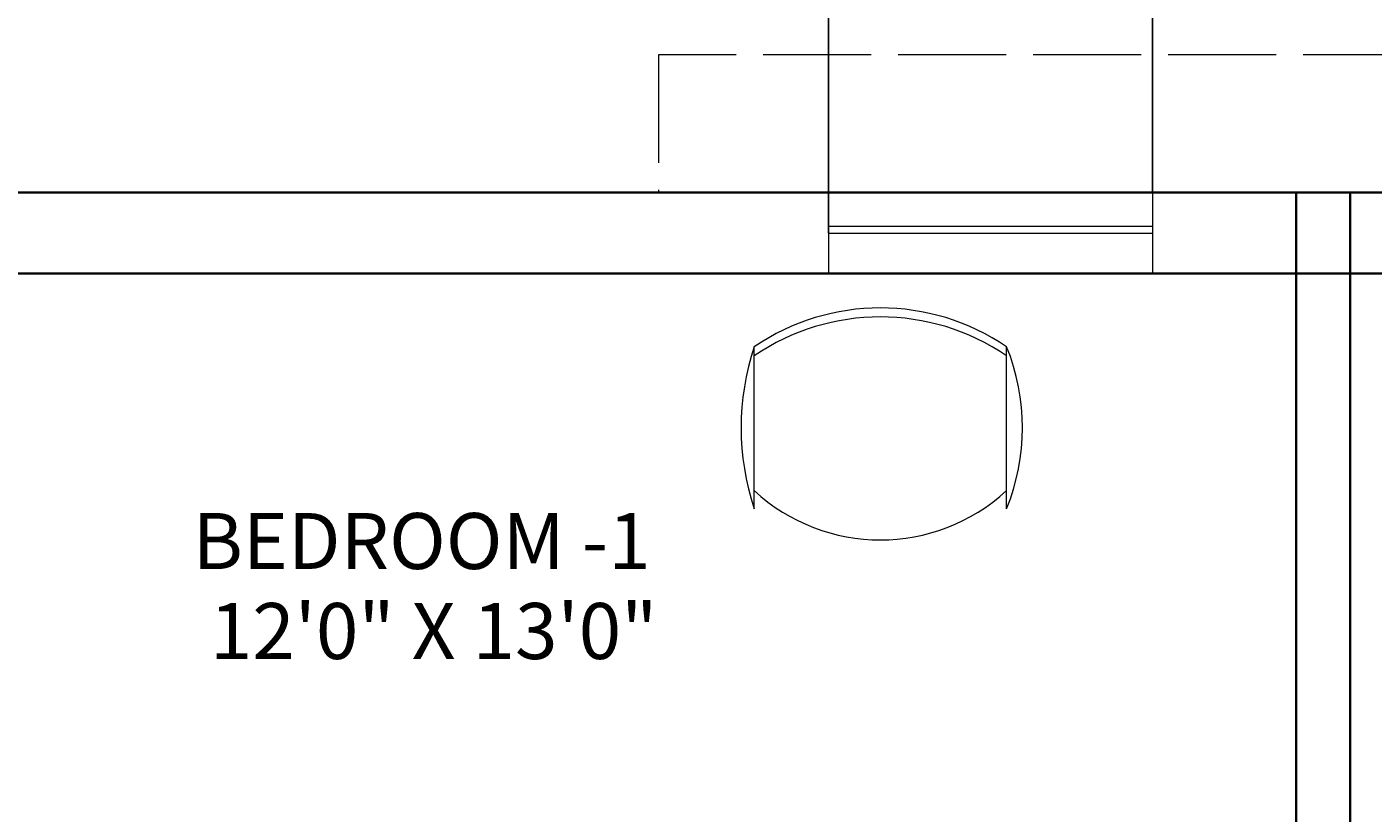
# Model space of a CAD drawing. Units: inches. Extents: x -61 to 1599, y -1316 to 257.
# Tile 41 of 204: x 91 to 240, y -686 to -599. Entities that reach past the tile are written whole.
import ezdxf

# ---------------------------------------------------------------- set-up
doc = ezdxf.new("R2010")
doc.units = ezdxf.units.IN
doc.header["$MEASUREMENT"] = 0
doc.linetypes.add('ACAD_ISO02W100', pattern=[15, 12, -3])
for name, color, linetype, lineweight in [('A-ANNO-DIMS', 2, 'Continuous', 18), ('A-AREA-IDEN', 1, 'Continuous', 18), ('A-FLOR-OVHD', 203, 'ACAD_ISO02W100', 13), ('FURNITURE', 83, 'Continuous', 18), ('WALLS', 4, 'Continuous', 35), ('WINDOWS', 220, 'Continuous', 18)]:
    doc.layers.add(name, color=color, linetype=linetype, lineweight=lineweight)
doc.styles.get("Standard").update_dxf_attribs({"font": 'arial.ttf'})
doc.dimstyles.get("Standard").update_dxf_attribs({"dimtxt": 0.18, "dimasz": 0.18, "dimexe": 0.18, "dimexo": 0.0625, "dimgap": 0.09, "dimtad": 0, "dimtih": 1, "dimtoh": 1, "dimdec": 0, "dimzin": 0, "dimdsep": 46, "dimlunit": 3, "dimtxsty": 'Standard', "dimcen": 0.09, "dimadec": 0, "dimazin": 0, "dimtfac": 1, "dimtdec": 0, "dimtofl": 0, "dimtmove": 0, "dimatfit": 3, "dimfxl": 1, "dimtolj": 1, "dimtzin": 0, "dimarcsym": 0})

# ---------------------------------------------------------------- blocks, each defined once
blk = doc.blocks.new('WIN-36IN')
for p, q in [((0, 4.5), (0, 9)), ((0, 9), (0, 0)), ((36, 9), (36, 0)), ((0, 5.26), (36, 5.26)), ((0, 4.5), (36, 4.5)), ((0, 4.5), (36, 4.5))]:
    blk.add_line(p, q)
blk = doc.blocks.new('BEDROOM-CHAIR')
for p, q in [((1.45, 3.47), (1.45, 21.47)), ((29.49, 3.47), (29.49, 21.47))]:
    blk.add_line(p, q)
for centre, radius, start, end in [((15.47, 0.83), 24.95, 55.8098, 124.1902), ((15.47, -0.17), 24.95, 55.8098, 124.1902), ((28.58, 12.47), 28.58, 161.6455, 198.3545), ((7.26, 12.47), 23.99, 337.9646, 22.0354), ((15.47, 20.69), 20.68, 227.332, 312.668)]:
    blk.add_arc(centre, radius, start, end)
blk = doc.blocks.new('*D687')
at = {"layer": 'A-ANNO-DIMS', "color": 0, "lineweight": -2, "transparency": 16777216}
for p, q in [((289.42, 181.68), (-61.08, 181.68)), ((-60.9, 181.5), (-60.9, -528.95)), ((-60.9, -1239.76), (-60.9, -529.32)), ((319.64, -1239.94), (-61.08, -1239.94))]:
    blk.add_line(p, q, dxfattribs=at)
at = {"layer": 'A-ANNO-DIMS', "color": 0, "transparency": 16777216}
for points in [[(-60.93, 181.5), (-60.87, 181.5), (-60.9, 181.68)], [(-60.93, -1239.76), (-60.87, -1239.76), (-60.9, -1239.94)]]:
    blk.add_solid(points, dxfattribs=at)
at = {"layer": 'DEFPOINTS', "color": 0, "transparency": 16777216}
for p in [(289.48, 181.68), (-60.9, -1239.94), (319.7, -1239.94)]:
    blk.add_point(p, dxfattribs=at)
at = {"layer": 'A-ANNO-DIMS', "color": 0, "transparency": 16777216, "insert": (-60.9, -529.13), "char_height": 0.18, "attachment_point": 5}
blk.add_mtext('\\A1;1421.6', dxfattribs=at)
blk = doc.blocks.new('*D700')
at = {"layer": 'A-ANNO-DIMS', "color": 0, "lineweight": -2, "transparency": 16777216}
for p, q in [((14.7, -616.88), (14.7, 257.46)), ((14.88, 257.28), (96.77, 257.28)), ((179.57, 257.28), (97.68, 257.28)), ((179.75, -616.88), (179.75, 257.46))]:
    blk.add_line(p, q, dxfattribs=at)
at = {"layer": 'A-ANNO-DIMS', "color": 0, "transparency": 16777216}
for points in [[(14.88, 257.31), (14.88, 257.25), (14.7, 257.28)], [(179.57, 257.31), (179.57, 257.25), (179.75, 257.28)]]:
    blk.add_solid(points, dxfattribs=at)
at = {"layer": 'DEFPOINTS', "color": 0, "transparency": 16777216}
for p in [(179.75, 257.28), (14.7, -616.94), (179.75, -616.94)]:
    blk.add_point(p, dxfattribs=at)
at = {"layer": 'A-ANNO-DIMS', "color": 0, "transparency": 16777216, "insert": (97.23, 257.28), "char_height": 0.18, "attachment_point": 5}
blk.add_mtext('\\A1;165.05', dxfattribs=at)
blk = doc.blocks.new('*D701')
at = {"layer": 'A-ANNO-DIMS', "color": 0, "lineweight": -2, "transparency": 16777216}
for p, q in [((215.75, -616.88), (215.75, 257.46)), ((215.93, 257.28), (233.92, 257.28)), ((252.7, 257.28), (234.71, 257.28)), ((252.88, -616.88), (252.88, 257.46))]:
    blk.add_line(p, q, dxfattribs=at)
at = {"layer": 'A-ANNO-DIMS', "color": 0, "transparency": 16777216}
for points in [[(215.93, 257.31), (215.93, 257.25), (215.75, 257.28)], [(252.7, 257.31), (252.7, 257.25), (252.88, 257.28)]]:
    blk.add_solid(points, dxfattribs=at)
at = {"layer": 'DEFPOINTS', "color": 0, "transparency": 16777216}
for p in [(252.88, 257.28), (215.75, -616.94), (252.88, -616.94)]:
    blk.add_point(p, dxfattribs=at)
at = {"layer": 'A-ANNO-DIMS', "color": 0, "transparency": 16777216, "insert": (234.32, 257.28), "char_height": 0.18, "attachment_point": 5}
blk.add_mtext('\\A1;37.13', dxfattribs=at)

msp = doc.modelspace()

# ---------------------------------------------------------------- linework, layer by layer
at = {"layer": 'A-FLOR-OVHD'}
for p, q in [((289.4807, -601.6522), (160.8585, -601.6522)), ((160.8585, -601.6522), (160.8585, -616.9446))]:
    msp.add_line(p, q, dxfattribs=at)
at = {"layer": 'WALLS'}
for p, q in [((544.7028, -616.9446), (14.7028, -616.9446)), ((231.7028, -616.9446), (231.7028, -787.9446)), ((237.7028, -616.9446), (237.7028, -787.9446)), ((87.7028, -625.9446), (231.7028, -625.9446)), ((231.7028, -625.9446), (237.7028, -625.9446)), ((237.7028, -625.9446), (321.7028, -625.9446))]:
    msp.add_line(p, q, dxfattribs=at)

# ---------------------------------------------------------------- block references
at = {"layer": 'FURNITURE'}
msp.add_blockref('BEDROOM-CHAIR', (170.039, -655.5427), dxfattribs=at)
at = {"layer": 'WINDOWS'}
msp.add_blockref('WIN-36IN', (179.752, -625.9447), dxfattribs=at)

# ---------------------------------------------------------------- texts
at = {"layer": 'A-AREA-IDEN'}
for s, height, p in [('BEDROOM -1', 6.22364, (109.1314, -658.7715)), (' 12\'0" X 13\'0"', 6.223643, (109.1314, -668.7692))]:
    msp.add_text(s, height=height, dxfattribs=at).set_placement(p)

# ---------------------------------------------------------------- dimensions: what is measured, and where the dimension line sits
at = {"layer": 'A-ANNO-DIMS'}
for base, p1, p2, picture, middle in [((179.7521, 257.2771), (14.7028, -616.9446), (179.7521, -616.9446), '*D700', (97.2274, 257.2771)), ((252.8825, 257.2771), (215.7521, -616.9446), (252.8825, -616.9446), '*D701', (234.3173, 257.2771))]:
    dim = msp.add_linear_dim(base=base, p1=p1, p2=p2, dimstyle='Standard', override={"dimdec": 2, "dimlfac": 1, "dimrnd": 0, "dimzin": 0, "dimdsep": 46, "dimlunit": 2}, dxfattribs=at)
    dim.commit()
    dim.dimension.update_dxf_attribs({"geometry": picture, "text_midpoint": middle})
dim = msp.add_linear_dim(base=(-60.8972, -1239.9446), p1=(289.4807, 181.6771), p2=(319.7028, -1239.9446), angle=90, dimstyle='Standard', override={"dimdec": 1, "dimlfac": 1, "dimrnd": 0, "dimzin": 0, "dimdsep": 46, "dimlunit": 2}, dxfattribs=at)
dim.commit()
dim.dimension.update_dxf_attribs({"geometry": '*D687', "text_midpoint": (-60.8972, -529.1337)})

doc.saveas('drawing.dxf')
